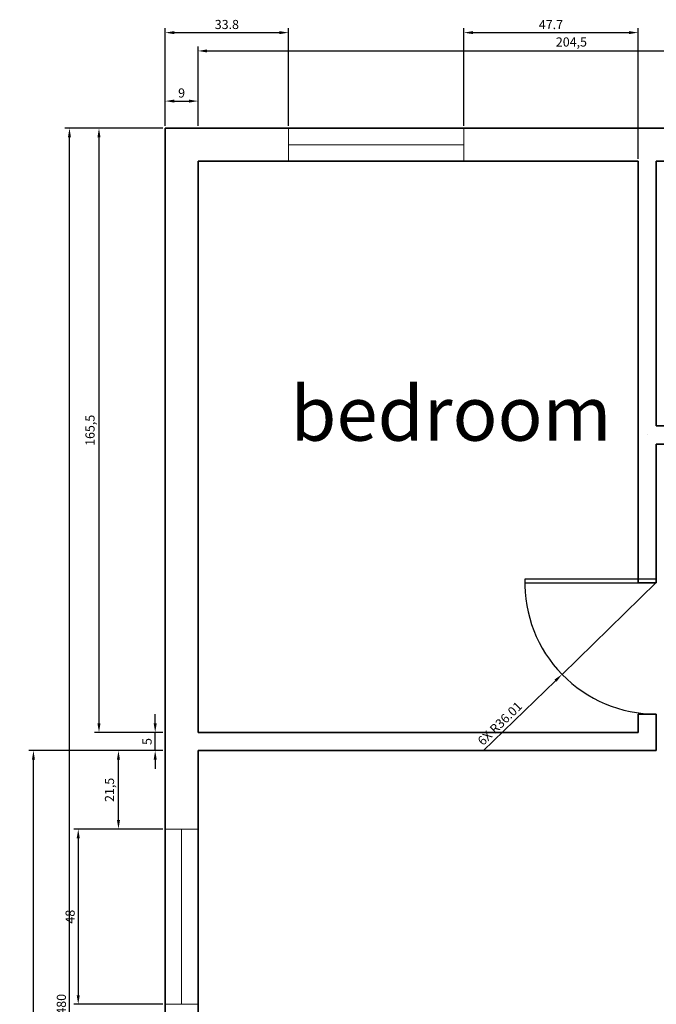
# Model space of a CAD drawing. Units: inches. Extents: x 64 to 791, y 453 to 990.
# Tile 2 of 3: x 357 to 531, y 721 to 990. Entities that reach past the tile are written whole.
import ezdxf

# ---------------------------------------------------------------- set-up
doc = ezdxf.new("R2010")
doc.units = ezdxf.units.IN
for name, color, linetype, lineweight in [('A-ANNO-DIMS', 2, 'Continuous', 18), ('A-AREA-IDEN', 7, 'Continuous', 25), ('A-DOOR', 3, 'Continuous', 25), ('A-GLAZ', 4, 'Continuous', 18), ('A-WALL', 7, 'Continuous', 35)]:
    doc.layers.add(name, color=color, linetype=linetype, lineweight=lineweight)
doc.styles.get("Standard").update_dxf_attribs({"font": 'arial.ttf'})
doc.dimstyles.new('ISO-25', dxfattribs={"dimtxt": 2.5, "dimasz": 2.5, "dimexe": 1.25, "dimexo": 0.625, "dimtad": 1, "dimtxsty": 'Standard', "dimcen": 2.5, "dimadec": 0, "dimazin": 0, "dimtfac": 1, "dimtmove": 0, "dimatfit": 3, "dimfxl": 1, "dimarcsym": 0})

# ---------------------------------------------------------------- blocks, each defined once
blk = doc.blocks.new('*D7')
at = {"layer": 'A-ANNO-DIMS', "color": 0, "lineweight": -2, "transparency": 16777216}
for p, q in [((405.94, 961.31), (405.94, 983.12)), ((408.44, 981.87), (607.94, 981.87)), ((610.44, 961.31), (610.44, 983.12))]:
    blk.add_line(p, q, dxfattribs=at)
at = {"layer": 'A-ANNO-DIMS', "color": 0, "transparency": 16777216}
for points in [[(408.44, 982.28), (408.44, 981.45), (405.94, 981.87)], [(607.94, 982.28), (607.94, 981.45), (610.44, 981.87)]]:
    blk.add_solid(points, dxfattribs=at)
at = {"layer": 'Defpoints', "color": 0, "transparency": 16777216}
for p in [(610.44, 981.87), (405.94, 960.68), (610.44, 960.68)]:
    blk.add_point(p, dxfattribs=at)
at = {"layer": 'A-ANNO-DIMS', "color": 0, "transparency": 16777216, "insert": (508.19, 984), "char_height": 2.5, "attachment_point": 5}
blk.add_mtext('204,5', dxfattribs=at)
blk = doc.blocks.new('*D8')
at = {"layer": 'A-ANNO-DIMS', "color": 0, "lineweight": -2, "transparency": 16777216}
for p, q in [((396.94, 961.31), (396.94, 969.38)), ((405.94, 961.31), (405.94, 969.38)), ((399.44, 968.13), (403.44, 968.13))]:
    blk.add_line(p, q, dxfattribs=at)
at = {"layer": 'A-ANNO-DIMS', "color": 0, "transparency": 16777216}
for points in [[(399.44, 968.54), (399.44, 967.71), (396.94, 968.13)], [(403.44, 968.54), (403.44, 967.71), (405.94, 968.13)]]:
    blk.add_solid(points, dxfattribs=at)
at = {"layer": 'Defpoints', "color": 0, "transparency": 16777216}
for p in [(405.94, 968.13), (396.94, 960.68), (405.94, 960.68)]:
    blk.add_point(p, dxfattribs=at)
at = {"layer": 'A-ANNO-DIMS', "color": 0, "transparency": 16777216, "insert": (401.44, 970.03), "char_height": 2.5, "attachment_point": 5}
blk.add_mtext('9', dxfattribs=at)
blk = doc.blocks.new('*D14')
at = {"layer": 'A-ANNO-DIMS', "color": 0, "lineweight": -2, "transparency": 16777216}
for p, q in [((396.31, 768.68), (371.89, 768.68)), ((373.14, 766.18), (373.14, 723.18)), ((396.31, 720.68), (371.89, 720.68))]:
    blk.add_line(p, q, dxfattribs=at)
at = {"layer": 'A-ANNO-DIMS', "color": 0, "transparency": 16777216}
for points in [[(372.72, 766.18), (373.55, 766.18), (373.14, 768.68)], [(372.72, 723.18), (373.55, 723.18), (373.14, 720.68)]]:
    blk.add_solid(points, dxfattribs=at)
at = {"layer": 'Defpoints', "color": 0, "transparency": 16777216}
for p in [(396.94, 768.68), (373.14, 720.68), (396.94, 720.68)]:
    blk.add_point(p, dxfattribs=at)
at = {"layer": 'A-ANNO-DIMS', "color": 0, "transparency": 16777216, "insert": (371.24, 744.68), "char_height": 2.5, "attachment_point": 5, "rotation": 90}
blk.add_mtext('48', dxfattribs=at)
blk = doc.blocks.new('*D19')
at = {"layer": 'A-ANNO-DIMS', "color": 0, "lineweight": -2, "transparency": 16777216}
for p, q in [((396.31, 960.68), (377.57, 960.68)), ((378.82, 958.18), (378.82, 797.68)), ((396.31, 795.18), (377.57, 795.18))]:
    blk.add_line(p, q, dxfattribs=at)
at = {"layer": 'A-ANNO-DIMS', "color": 0, "transparency": 16777216}
for points in [[(378.4, 958.18), (379.24, 958.18), (378.82, 960.68)], [(378.4, 797.68), (379.24, 797.68), (378.82, 795.18)]]:
    blk.add_solid(points, dxfattribs=at)
at = {"layer": 'Defpoints', "color": 0, "transparency": 16777216}
for p in [(396.94, 960.68), (378.82, 795.18), (396.94, 795.18)]:
    blk.add_point(p, dxfattribs=at)
at = {"layer": 'A-ANNO-DIMS', "color": 0, "transparency": 16777216, "insert": (376.69, 877.93), "char_height": 2.5, "attachment_point": 5, "rotation": 90}
blk.add_mtext('165,5', dxfattribs=at)
blk = doc.blocks.new('*D20')
at = {"layer": 'A-ANNO-DIMS', "color": 0, "lineweight": -2, "transparency": 16777216}
for p, q in [((394.21, 797.68), (394.21, 800.18)), ((396.31, 795.18), (392.96, 795.18)), ((394.21, 790.18), (394.21, 795.18)), ((396.31, 790.18), (392.96, 790.18)), ((394.21, 787.68), (394.21, 785.18))]:
    blk.add_line(p, q, dxfattribs=at)
at = {"layer": 'A-ANNO-DIMS', "color": 0, "transparency": 16777216}
for points in [[(393.79, 797.68), (394.63, 797.68), (394.21, 795.18)], [(393.79, 787.68), (394.63, 787.68), (394.21, 790.18)]]:
    blk.add_solid(points, dxfattribs=at)
at = {"layer": 'Defpoints', "color": 0, "transparency": 16777216}
for p in [(394.21, 795.18), (396.94, 795.18), (396.94, 790.18)]:
    blk.add_point(p, dxfattribs=at)
at = {"layer": 'A-ANNO-DIMS', "color": 0, "transparency": 16777216, "insert": (392.31, 792.68), "char_height": 2.5, "attachment_point": 5, "rotation": 90}
blk.add_mtext('5', dxfattribs=at)
blk = doc.blocks.new('*D21')
at = {"layer": 'A-ANNO-DIMS', "color": 0, "lineweight": -2, "transparency": 16777216}
for p, q in [((396.31, 790.18), (382.9, 790.18)), ((384.15, 771.18), (384.15, 787.68)), ((396.31, 768.68), (382.9, 768.68))]:
    blk.add_line(p, q, dxfattribs=at)
at = {"layer": 'A-ANNO-DIMS', "color": 0, "transparency": 16777216}
for points in [[(383.73, 787.68), (384.57, 787.68), (384.15, 790.18)], [(383.73, 771.18), (384.57, 771.18), (384.15, 768.68)]]:
    blk.add_solid(points, dxfattribs=at)
at = {"layer": 'Defpoints', "color": 0, "transparency": 16777216}
for p in [(384.15, 790.18), (396.94, 790.18), (396.94, 768.68)]:
    blk.add_point(p, dxfattribs=at)
at = {"layer": 'A-ANNO-DIMS', "color": 0, "transparency": 16777216, "insert": (382.02, 779.43), "char_height": 2.5, "attachment_point": 5, "rotation": 90}
blk.add_mtext('21,5', dxfattribs=at)
blk = doc.blocks.new('*D22')
at = {"layer": 'A-ANNO-DIMS', "color": 0, "lineweight": -2, "transparency": 16777216}
for p, q in [((396.31, 790.18), (359.63, 790.18)), ((360.88, 483.18), (360.88, 787.68)), ((396.31, 480.68), (359.63, 480.68))]:
    blk.add_line(p, q, dxfattribs=at)
at = {"layer": 'A-ANNO-DIMS', "color": 0, "transparency": 16777216}
for points in [[(360.46, 787.68), (361.29, 787.68), (360.88, 790.18)], [(360.46, 483.18), (361.29, 483.18), (360.88, 480.68)]]:
    blk.add_solid(points, dxfattribs=at)
at = {"layer": 'Defpoints', "color": 0, "transparency": 16777216}
for p in [(360.88, 790.18), (396.94, 790.18), (396.94, 480.68)]:
    blk.add_point(p, dxfattribs=at)
at = {"layer": 'A-ANNO-DIMS', "color": 0, "transparency": 16777216, "insert": (358.75, 635.43), "char_height": 2.5, "attachment_point": 5, "rotation": 90}
blk.add_mtext('309,5', dxfattribs=at)
blk = doc.blocks.new('WIN-48IN')
for p, q in [((0, 48), (9, 48)), ((4.5, 48), (4.5, 0)), ((0, 0), (9, 0))]:
    blk.add_line(p, q)
blk = doc.blocks.new('DOOR-SWING-36IN')
for p, q in [((0, 0), (0, 5)), ((36, 0), (36, 5))]:
    blk.add_line(p, q)
blk.add_lwpolyline([(36, 0), (37, 0), (37, 36), (36, 36)], close=True)
blk.add_arc((36.01, 0), 36.01, 88.4304, 180)
blk = doc.blocks.new('*D33')
at = {"layer": 'A-ANNO-DIMS', "color": 0, "lineweight": -2, "transparency": 16777216}
for p, q in [((396.31, 960.68), (369.49, 960.68)), ((370.74, 483.18), (370.74, 958.18)), ((396.31, 480.68), (369.49, 480.68))]:
    blk.add_line(p, q, dxfattribs=at)
at = {"layer": 'A-ANNO-DIMS', "color": 0, "transparency": 16777216}
for points in [[(370.32, 958.18), (371.15, 958.18), (370.74, 960.68)], [(370.32, 483.18), (371.15, 483.18), (370.74, 480.68)]]:
    blk.add_solid(points, dxfattribs=at)
at = {"layer": 'Defpoints', "color": 0, "transparency": 16777216}
for p in [(370.74, 960.68), (396.94, 960.68), (396.94, 480.68)]:
    blk.add_point(p, dxfattribs=at)
at = {"layer": 'A-ANNO-DIMS', "color": 0, "transparency": 16777216, "insert": (368.84, 720.68), "char_height": 2.5, "attachment_point": 5, "rotation": 90}
blk.add_mtext('480', dxfattribs=at)
blk = doc.blocks.new('*D34')
at = {"layer": 'A-ANNO-DIMS', "color": 0, "lineweight": -2, "transparency": 16777216}
for p, q in [((478.74, 961.31), (478.74, 988.13)), ((526.44, 952.31), (526.44, 988.13)), ((481.24, 986.88), (523.94, 986.88))]:
    blk.add_line(p, q, dxfattribs=at)
at = {"layer": 'A-ANNO-DIMS', "color": 0, "transparency": 16777216}
for points in [[(481.24, 987.3), (481.24, 986.47), (478.74, 986.88)], [(523.94, 987.3), (523.94, 986.47), (526.44, 986.88)]]:
    blk.add_solid(points, dxfattribs=at)
at = {"layer": 'Defpoints', "color": 0, "transparency": 16777216}
for p in [(526.44, 986.88), (478.74, 960.68), (526.44, 951.68)]:
    blk.add_point(p, dxfattribs=at)
at = {"layer": 'A-ANNO-DIMS', "color": 0, "transparency": 16777216, "insert": (502.59, 988.76), "char_height": 2.5, "attachment_point": 5}
blk.add_mtext('47.7', dxfattribs=at)
blk = doc.blocks.new('*D37')
at = {"layer": 'A-ANNO-DIMS', "color": 0, "lineweight": -2, "transparency": 16777216}
for p, q in [((396.94, 961.31), (396.94, 988.13)), ((430.74, 961.31), (430.74, 988.13)), ((399.44, 986.88), (428.24, 986.88))]:
    blk.add_line(p, q, dxfattribs=at)
at = {"layer": 'A-ANNO-DIMS', "color": 0, "transparency": 16777216}
for points in [[(399.44, 987.3), (399.44, 986.47), (396.94, 986.88)], [(428.24, 987.3), (428.24, 986.47), (430.74, 986.88)]]:
    blk.add_solid(points, dxfattribs=at)
at = {"layer": 'Defpoints', "color": 0, "transparency": 16777216}
for p in [(430.74, 986.88), (396.94, 960.68), (430.74, 960.68)]:
    blk.add_point(p, dxfattribs=at)
at = {"layer": 'A-ANNO-DIMS', "color": 0, "transparency": 16777216, "insert": (413.84, 988.79), "char_height": 2.5, "attachment_point": 5}
blk.add_mtext('33.8', dxfattribs=at)
blk = doc.blocks.new('*D55')
at = {"layer": 'A-ANNO-DIMS', "color": 0, "lineweight": -2, "transparency": 16777216}
for p, q in [((531.44, 836.2), (505.62, 811.08)), ((484.05, 790.09), (503.83, 809.34))]:
    blk.add_line(p, q, dxfattribs=at)
at = {"layer": 'A-ANNO-DIMS', "color": 0, "transparency": 16777216}
blk.add_solid([(503.54, 809.64), (504.12, 809.04), (505.62, 811.08)], dxfattribs=at)
at = {"layer": 'Defpoints', "color": 0, "transparency": 16777216}
for p in [(531.44, 836.2), (505.62, 811.08)]:
    blk.add_point(p, dxfattribs=at)
at = {"layer": 'A-ANNO-DIMS', "color": 0, "transparency": 16777216, "insert": (488.81, 797.38), "char_height": 2.5, "attachment_point": 5, "rotation": 44.2145}
blk.add_mtext('6X R36.01', dxfattribs=at)

msp = doc.modelspace()

# ---------------------------------------------------------------- linework, layer by layer
at = {"layer": 'A-WALL'}
for p, q in [((756.937, 960.6832), (396.937, 960.6832)), ((396.937, 960.6832), (396.937, 480.6832)), ((396.937, 960.6832), (528.937, 960.6832)), ((528.937, 960.6832), (612.937, 960.6832)), ((405.937, 951.6832), (526.437, 951.6832)), ((405.937, 951.6832), (405.937, 795.1832)), ((526.437, 951.6832), (405.937, 951.6832)), ((526.437, 951.6832), (526.437, 836.1832)), ((531.437, 951.6832), (531.437, 879.1832)), ((610.437, 951.6832), (531.437, 951.6832)), ((528.937, 876.6832), (528.937, 876.6832)), ((571.437, 879.1832), (531.437, 879.1832)), ((531.437, 874.1832), (531.437, 836.1832)), ((571.437, 874.1832), (531.437, 874.1832)), ((526.437, 836.1832), (531.437, 836.1832)), ((526.437, 800.1832), (531.437, 800.1832)), ((526.437, 800.1832), (526.437, 795.1832)), ((531.437, 800.1832), (531.437, 790.1832)), ((405.937, 795.1832), (526.437, 795.1832)), ((405.937, 790.1832), (531.437, 790.1832)), ((405.937, 790.1832), (405.937, 567.1832))]:
    msp.add_line(p, q, dxfattribs=at)

# ---------------------------------------------------------------- block references
at = {"layer": 'A-DOOR', "rotation": 89.99999999999966}
msp.add_blockref('DOOR-SWING-36IN', (531.4372, 800.1832), dxfattribs=at)
at = {"layer": 'A-GLAZ', "rotation": 269.9999999999999}
msp.add_blockref('WIN-48IN', (430.7361, 960.6832), dxfattribs=at)
at = {"layer": 'A-GLAZ'}
msp.add_blockref('WIN-48IN', (396.937, 720.6828), dxfattribs=at)

# ---------------------------------------------------------------- texts
at = {"layer": 'A-AREA-IDEN'}
msp.add_text('bedroom ', height=14.92404, dxfattribs=at).set_placement((431.2544, 875.0819))

# ---------------------------------------------------------------- dimensions: what is measured, and where the dimension line sits
at = {"layer": 'A-ANNO-DIMS'}
for base, p1, p2, override, picture, middle in [((430.7365, 986.8832), (396.937, 960.6832), (430.7365, 960.6832), {"dimdec": 1, "dimlfac": 1, "dimrnd": 0, "dimzin": 0, "dimdsep": 46, "dimlunit": 2}, '*D37', (413.8367, 988.7855)), ((526.437, 986.8832), (478.7365, 960.6832), (526.437, 951.6832), {"dimdec": 1, "dimlfac": 1, "dimrnd": 0, "dimzin": 0, "dimdsep": 46, "dimlunit": 2}, '*D34', (502.5867, 988.7582)), ((610.437, 981.8679), (405.937, 960.6832), (610.437, 960.6832), {"dimclrd": 0, "dimclre": 0, "dimclrt": 0}, '*D7', (508.187, 983.9953)), ((405.937, 968.1276), (396.937, 960.6832), (405.937, 960.6832), {"dimclrd": 0, "dimclre": 0, "dimclrt": 0}, '*D8', (401.437, 970.029))]:
    dim = msp.add_linear_dim(base=base, p1=p1, p2=p2, dimstyle='ISO-25', override=override, dxfattribs=at)
    dim.commit()
    dim.dimension.update_dxf_attribs({"geometry": picture, "text_midpoint": middle})
for base, p1, p2, override, picture, middle in [((370.737, 960.6832), (396.937, 480.6832), (396.937, 960.6832), {"dimdec": 0, "dimlfac": 1, "dimrnd": 0, "dimzin": 0, "dimdsep": 46, "dimlunit": 2}, '*D33', (368.8355, 720.6832)), ((378.8213, 795.1832), (396.937, 960.6832), (396.937, 795.1832), {"dimclrd": 0, "dimclre": 0, "dimclrt": 0}, '*D19', (376.6939, 877.9332)), ((394.2086, 795.1832), (396.937, 790.1832), (396.937, 795.1832), {"dimclrd": 0, "dimclre": 0, "dimclrt": 0}, '*D20', (392.3122, 792.6832)), ((360.8763, 790.1832), (396.937, 480.6832), (396.937, 790.1832), {"dimclrd": 0, "dimclre": 0, "dimclrt": 0}, '*D22', (358.749, 635.4332)), ((384.1511, 790.1832), (396.937, 768.6832), (396.937, 790.1832), {"dimclrd": 0, "dimclre": 0, "dimclrt": 0}, '*D21', (382.0237, 779.4332)), ((373.1367, 720.6832), (396.937, 768.6832), (396.937, 720.6832), {"dimclrd": 0, "dimclre": 0, "dimclrt": 0}, '*D14', (371.2352, 744.6832))]:
    dim = msp.add_linear_dim(base=base, p1=p1, p2=p2, angle=90, dimstyle='ISO-25', override=override, dxfattribs=at)
    dim.commit()
    dim.dimension.update_dxf_attribs({"geometry": picture, "text_midpoint": middle})
dim = msp.add_radius_dim(center=(531.437, 836.1967), mpoint=(505.6248, 811.0828), text='6X <>', dimstyle='ISO-25', override={"dimdec": 2, "dimlfac": 1, "dimrnd": 0, "dimzin": 0, "dimdsep": 46, "dimlunit": 2}, dxfattribs=at)
dim.commit()
dim.dimension.update_dxf_attribs({"geometry": '*D55', "text_midpoint": (490.1376, 796.0145), "dimtype": 164})

doc.saveas('drawing.dxf')
